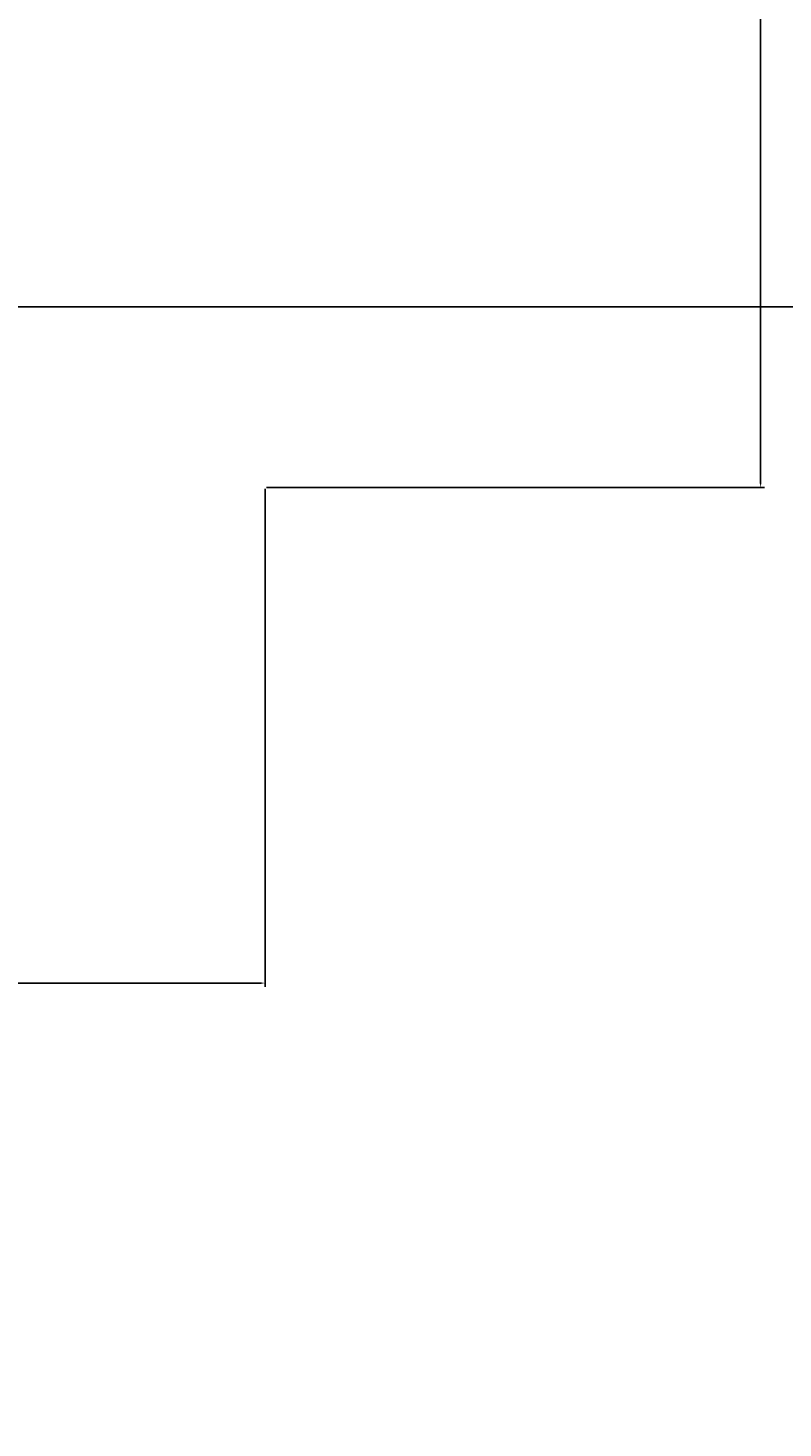
# Model space of a CAD drawing. Units: inches. Extents: x 182 to 1022, y -617 to 111.
# Tile 12 of 33: x 399 to 433, y -340 to -276. Entities that reach past the tile are written whole.
import ezdxf

# ---------------------------------------------------------------- set-up
doc = ezdxf.new("R2010")
doc.units = ezdxf.units.IN
doc.header["$MEASUREMENT"] = 0
doc.layers.add('A-ANNO-DIMS', color=2, linetype='Continuous', lineweight=18)
doc.styles.get("Standard").update_dxf_attribs({"font": 'arial.ttf'})
doc.dimstyles.get("Standard").update_dxf_attribs({"dimtxt": 0.18, "dimasz": 0.18, "dimexe": 0.18, "dimexo": 0.0625, "dimgap": 0.09, "dimtad": 0, "dimtih": 1, "dimtoh": 1, "dimdec": 1, "dimzin": 0, "dimdsep": 46, "dimlunit": 4, "dimtxsty": 'Standard', "dimcen": 0.09, "dimadec": 0, "dimazin": 0, "dimtfac": 1, "dimtdec": 1, "dimtofl": 0, "dimtmove": 0, "dimatfit": 3, "dimfxl": 1, "dimtolj": 1, "dimtzin": 0, "dimarcsym": 0})

# ---------------------------------------------------------------- blocks, each defined once
blk = doc.blocks.new('*D26')
at = {"layer": 'A-ANNO-DIMS', "color": 0, "lineweight": -2, "transparency": 16777216}
for p, q in [((257.848, -296.884), (257.848, -319.733)), ((409.388, -296.884), (409.388, -319.733)), ((258.028, -319.553), (331.642, -319.553)), ((409.208, -319.553), (335.594, -319.553))]:
    blk.add_line(p, q, dxfattribs=at)
at = {"layer": 'A-ANNO-DIMS', "color": 0, "transparency": 16777216}
for points in [[(258.028, -319.523), (258.028, -319.583), (257.848, -319.553)], [(409.208, -319.523), (409.208, -319.583), (409.388, -319.553)]]:
    blk.add_solid(points, dxfattribs=at)
at = {"layer": 'Defpoints', "color": 0, "transparency": 16777216}
for p in [(257.848, -296.822), (409.388, -296.822), (409.388, -319.553)]:
    blk.add_point(p, dxfattribs=at)
at = {"layer": 'A-ANNO-DIMS', "color": 0, "transparency": 16777216, "insert": (333.618, -319.553), "char_height": 0.18, "attachment_point": 5}
blk.add_mtext('\\A1;LOUNGE GROUP 12\'-7 1/2" TYP.', dxfattribs=at)
blk = doc.blocks.new('*D27')
at = {"layer": 'A-ANNO-DIMS', "color": 0, "lineweight": -2, "transparency": 16777216}
for p, q in [((409.45, -214.092), (432.299, -214.092)), ((432.119, -214.272), (432.119, -255.274)), ((432.119, -296.642), (432.119, -255.64)), ((409.45, -296.822), (432.299, -296.822))]:
    blk.add_line(p, q, dxfattribs=at)
at = {"layer": 'A-ANNO-DIMS', "color": 0, "transparency": 16777216}
for points in [[(432.089, -214.272), (432.149, -214.272), (432.119, -214.092)], [(432.089, -296.642), (432.149, -296.642), (432.119, -296.822)]]:
    blk.add_solid(points, dxfattribs=at)
at = {"layer": 'Defpoints', "color": 0, "transparency": 16777216}
for p in [(409.388, -214.092), (432.119, -214.092), (409.388, -296.822)]:
    blk.add_point(p, dxfattribs=at)
at = {"layer": 'A-ANNO-DIMS', "color": 0, "transparency": 16777216, "insert": (432.119, -255.457), "char_height": 0.18, "attachment_point": 5}
blk.add_mtext('\\A1;6\'-10 1/2" TYP.', dxfattribs=at)
blk = doc.blocks.new('*D39')
at = {"layer": 'A-ANNO-DIMS', "color": 0, "lineweight": -2, "transparency": 16777216}
for p, q in [((238.398, -288.54), (1015.285, -288.54)), ((1015.105, -288.72), (1015.105, -346.775)), ((1015.105, -405.193), (1015.105, -347.138)), ((238.427, -405.373), (1015.285, -405.373))]:
    blk.add_line(p, q, dxfattribs=at)
at = {"layer": 'A-ANNO-DIMS', "color": 0, "transparency": 16777216}
for points in [[(1015.075, -288.72), (1015.135, -288.72), (1015.105, -288.54)], [(1015.075, -405.193), (1015.135, -405.193), (1015.105, -405.373)]]:
    blk.add_solid(points, dxfattribs=at)
at = {"layer": 'Defpoints', "color": 0, "transparency": 16777216}
for p in [(238.335, -288.54), (1015.105, -288.54), (238.364, -405.373)]:
    blk.add_point(p, dxfattribs=at)
at = {"layer": 'A-ANNO-DIMS', "color": 0, "transparency": 16777216, "insert": (1015.105, -346.956), "char_height": 0.18, "attachment_point": 5}
blk.add_mtext('\\A1;9\'-9"', dxfattribs=at)

msp = doc.modelspace()

# ---------------------------------------------------------------- dimensions: what is measured, and where the dimension line sits
at = {"layer": 'A-ANNO-DIMS'}
dim = msp.add_linear_dim(base=(432.119, -214.092), p1=(409.388, -296.822), p2=(409.388, -214.092), angle=90, text='<> TYP.', dimstyle='Standard', override={"dimdec": 1, "dimlfac": 1, "dimrnd": 0, "dimzin": 1, "dimdsep": 46, "dimlunit": 4, "dimfrac": 2}, dxfattribs=at)
dim.commit()
dim.dimension.update_dxf_attribs({"geometry": '*D27', "text_midpoint": (432.119, -255.457)})
dim = msp.add_linear_dim(base=(1015.105, -288.54), p1=(238.364, -405.373), p2=(238.335, -288.54), angle=90, dimstyle='Standard', override={"dimdec": 1, "dimlfac": 1, "dimrnd": 0, "dimzin": 1, "dimdsep": 46, "dimlunit": 4, "dimfrac": 2}, dxfattribs=at)
dim.commit()
dim.dimension.update_dxf_attribs({"geometry": '*D39', "text_midpoint": (1015.105, -346.956)})
dim = msp.add_linear_dim(base=(409.388, -319.553), p1=(257.848, -296.822), p2=(409.388, -296.822), text='LOUNGE GROUP <> TYP.', dimstyle='Standard', override={"dimdec": 1, "dimlfac": 1, "dimrnd": 0, "dimzin": 1, "dimdsep": 46, "dimlunit": 4, "dimfrac": 2}, dxfattribs=at)
dim.commit()
dim.dimension.update_dxf_attribs({"geometry": '*D26', "text_midpoint": (333.618, -319.553)})

doc.saveas('drawing.dxf')
